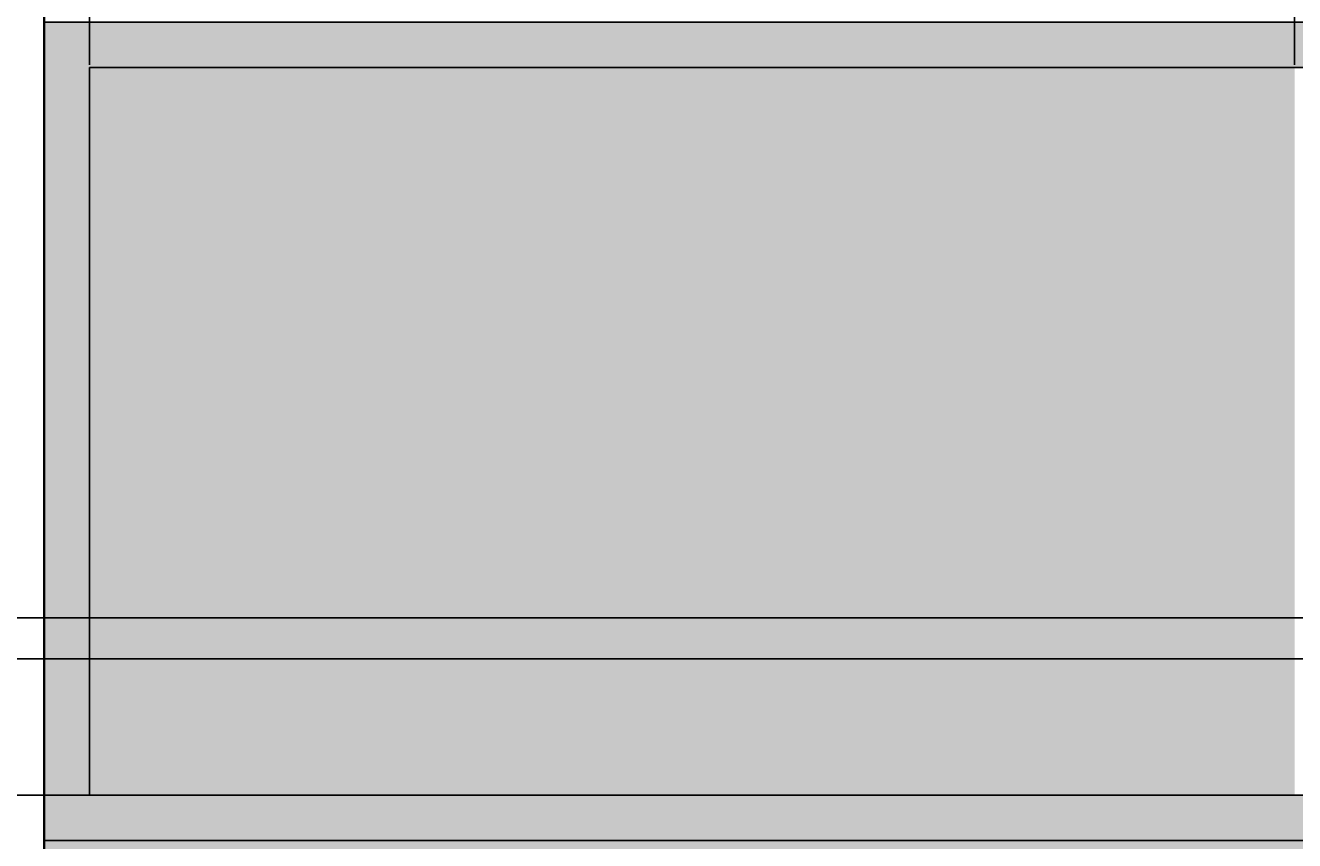
# Model space of a CAD drawing. Units: inches. Extents: x 4508 to 4723, y 847 to 1020.
# Tile 3 of 32: x 4550 to 4577, y 887 to 905. Entities that reach past the tile are written whole.
import ezdxf

# ---------------------------------------------------------------- set-up
doc = ezdxf.new("R2010")
doc.units = ezdxf.units.IN
for name, color, linetype, lineweight in [('A-ANNO-DIMS', 2, 'Continuous', 18), ('A-FURN', 8, 'Continuous', 25), ('A-WALL', 7, 'Continuous', 35), ('A-WALL-PATT', 254, 'Continuous', 13)]:
    doc.layers.add(name, color=color, linetype=linetype, lineweight=lineweight)
doc.styles.get("Standard").update_dxf_attribs({"font": 'arial.ttf'})
doc.dimstyles.get("Standard").update_dxf_attribs({"dimtxt": 0.18, "dimasz": 0.18, "dimexe": 0.18, "dimexo": 0.0625, "dimgap": 0.09, "dimtad": 0, "dimtih": 1, "dimtoh": 1, "dimdec": 4, "dimzin": 0, "dimdsep": 46, "dimtxsty": 'Standard', "dimcen": 0.09, "dimadec": 0, "dimazin": 0, "dimtfac": 1, "dimtdec": 4, "dimtofl": 0, "dimtmove": 0, "dimatfit": 3, "dimfxl": 1, "dimtolj": 1, "dimtzin": 0, "dimarcsym": 0})

# ---------------------------------------------------------------- blocks, each defined once
blk = doc.blocks.new('*D26')
at = {"layer": 'A-ANNO-DIMS', "color": 0, "lineweight": -2, "transparency": 16777216}
for p, q in [((4549.994, 904.809), (4549.994, 1002.877)), ((4550.994, 903.809), (4550.994, 1002.877)), ((4550.174, 1002.697), (4550.371, 1002.697)), ((4550.814, 1002.697), (4550.617, 1002.697))]:
    blk.add_line(p, q, dxfattribs=at)
at = {"layer": 'A-ANNO-DIMS', "color": 0, "lineweight": 9, "transparency": 16777216}
for points in [[(4550.174, 1002.727), (4550.174, 1002.667), (4549.994, 1002.697)], [(4550.814, 1002.727), (4550.814, 1002.667), (4550.994, 1002.697)]]:
    blk.add_solid(points, dxfattribs=at)
at = {"layer": 'Defpoints', "color": 0, "lineweight": 9, "transparency": 16777216}
for p in [(4550.994, 1002.697), (4549.994, 904.747), (4550.994, 903.747)]:
    blk.add_point(p, dxfattribs=at)
at = {"layer": 'A-ANNO-DIMS', "color": 0, "transparency": 16777216, "insert": (4550.494, 1002.697), "char_height": 0.18, "attachment_point": 5}
blk.add_mtext('\\A1;1', dxfattribs=at)
blk = doc.blocks.new('*D27')
at = {"layer": 'A-ANNO-DIMS', "color": 0, "lineweight": -2, "transparency": 16777216}
for p, q in [((4550.994, 903.809), (4550.994, 1002.877)), ((4577.494, 903.809), (4577.494, 1002.877)), ((4551.174, 1002.697), (4563.918, 1002.697)), ((4577.314, 1002.697), (4564.57, 1002.697))]:
    blk.add_line(p, q, dxfattribs=at)
at = {"layer": 'A-ANNO-DIMS', "color": 0, "lineweight": 9, "transparency": 16777216}
for points in [[(4551.174, 1002.727), (4551.174, 1002.667), (4550.994, 1002.697)], [(4577.314, 1002.727), (4577.314, 1002.667), (4577.494, 1002.697)]]:
    blk.add_solid(points, dxfattribs=at)
at = {"layer": 'Defpoints', "color": 0, "lineweight": 9, "transparency": 16777216}
for p in [(4577.494, 1002.697), (4550.994, 903.747), (4577.494, 903.747)]:
    blk.add_point(p, dxfattribs=at)
at = {"layer": 'A-ANNO-DIMS', "color": 0, "transparency": 16777216, "insert": (4564.244, 1002.697), "char_height": 0.18, "attachment_point": 5}
blk.add_mtext('\\A1;26.5', dxfattribs=at)
blk = doc.blocks.new('*D28')
at = {"layer": 'A-ANNO-DIMS', "color": 0, "lineweight": -2, "transparency": 16777216}
for p, q in [((4577.494, 903.809), (4577.494, 1002.877)), ((4577.994, 903.809), (4577.994, 1002.877)), ((4577.314, 1002.697), (4577.134, 1002.697)), ((4578.174, 1002.697), (4578.354, 1002.697))]:
    blk.add_line(p, q, dxfattribs=at)
at = {"layer": 'A-ANNO-DIMS', "color": 0, "lineweight": 9, "transparency": 16777216}
for points in [[(4577.314, 1002.727), (4577.314, 1002.667), (4577.494, 1002.697)], [(4578.174, 1002.727), (4578.174, 1002.667), (4577.994, 1002.697)]]:
    blk.add_solid(points, dxfattribs=at)
at = {"layer": 'Defpoints', "color": 0, "lineweight": 9, "transparency": 16777216}
for p in [(4577.994, 1002.697), (4577.494, 903.747), (4577.994, 903.747)]:
    blk.add_point(p, dxfattribs=at)
at = {"layer": 'A-ANNO-DIMS', "color": 0, "transparency": 16777216, "insert": (4578.608, 1002.697), "char_height": 0.18, "attachment_point": 5}
blk.add_mtext('\\A1;0.5', dxfattribs=at)
blk = doc.blocks.new('*D32')
at = {"layer": 'A-ANNO-DIMS', "color": 0, "lineweight": -2, "transparency": 16777216}
for p, q in [((4604.431, 890.747), (4532.864, 890.747)), ((4533.044, 890.567), (4533.044, 889.429)), ((4533.044, 887.927), (4533.044, 889.065)), ((4604.431, 887.747), (4532.864, 887.747))]:
    blk.add_line(p, q, dxfattribs=at)
at = {"layer": 'A-ANNO-DIMS', "color": 0, "lineweight": 9, "transparency": 16777216}
for points in [[(4533.014, 890.567), (4533.074, 890.567), (4533.044, 890.747)], [(4533.014, 887.927), (4533.074, 887.927), (4533.044, 887.747)]]:
    blk.add_solid(points, dxfattribs=at)
at = {"layer": 'Defpoints', "color": 0, "lineweight": 9, "transparency": 16777216}
for p in [(4533.044, 890.747), (4604.494, 890.747), (4604.494, 887.747)]:
    blk.add_point(p, dxfattribs=at)
at = {"layer": 'A-ANNO-DIMS', "color": 0, "transparency": 16777216, "insert": (4533.044, 889.247), "char_height": 0.18, "attachment_point": 5}
blk.add_mtext('\\A1;3', dxfattribs=at)
blk = doc.blocks.new('*D41')
at = {"layer": 'A-ANNO-DIMS', "color": 0, "lineweight": -2, "transparency": 16777216}
for p, q in [((4533.044, 891.643), (4533.044, 891.823)), ((4533.044, 891.823), (4533.224, 891.823)), ((4616.47, 891.643), (4532.864, 891.643)), ((4533.044, 890.927), (4533.044, 891.463)), ((4608.499, 890.747), (4532.864, 890.747))]:
    blk.add_line(p, q, dxfattribs=at)
at = {"layer": 'A-ANNO-DIMS', "color": 0, "lineweight": 9, "transparency": 16777216}
for points in [[(4533.014, 891.463), (4533.074, 891.463), (4533.044, 891.643)], [(4533.014, 890.927), (4533.074, 890.927), (4533.044, 890.747)]]:
    blk.add_solid(points, dxfattribs=at)
at = {"layer": 'Defpoints', "color": 0, "lineweight": 9, "transparency": 16777216}
for p in [(4533.044, 891.643), (4616.533, 891.643), (4608.562, 890.747)]:
    blk.add_point(p, dxfattribs=at)
at = {"layer": 'A-ANNO-DIMS', "color": 0, "transparency": 16777216, "insert": (4533.547, 891.823), "char_height": 0.18, "attachment_point": 5}
blk.add_mtext('\\A1;0.90', dxfattribs=at)

msp = doc.modelspace()

# ---------------------------------------------------------------- hatches: boundary and pattern name
at = {"layer": 'A-WALL-PATT', "transparency": 33554508}
h = msp.add_hatch(color=256, dxfattribs=at)
h.dxf.hatch_style = 1
h.paths.add_polyline_path([(4661.6706, 954.043, -0.3739004), (4658.5765, 957.6021, -1), (4665.7646, 957.6021, -0.3739004), (4662.6706, 954.043), (4662.6706, 944.4021, -0.2114781), (4670.3062, 945.0869), (4670.3062, 968.0592, -0.4632086), (4663.3246, 973.9783, -0.4632086), (4670.3062, 979.8975), (4670.3062, 994.7469), (4588.9938, 994.7469), (4588.9938, 904.7469), (4657.9938, 904.7469), (4657.9938, 886.7469), (4549.9938, 886.7469), (4549.9938, 878.7469), (4693.9938, 878.7469), (4693.9938, 994.7469), (4671.8062, 994.7469), (4671.8062, 979.4411, -0.2941682), (4675.3246, 973.9783, -0.2941682), (4671.8062, 968.5156), (4671.8062, 944.4278, -0.2741114), (4676.7298, 936.1217, -0.2741114), (4671.8062, 927.8155), (4671.8062, 907.6998, -0.3779645), (4677.0562, 901.7469, -0.3779645), (4671.8062, 895.7939), (4671.8062, 883.7469), (4670.3062, 883.7469), (4670.3062, 895.7939, -0.3779645), (4665.0562, 901.7469, -0.3779645), (4670.3062, 907.6998), (4670.3062, 927.1564, -0.2114781), (4662.6706, 927.8412), (4662.6706, 918.2003, -0.3739004), (4665.7646, 914.6412, -1), (4658.5765, 914.6412, -0.3739004), (4661.6706, 918.2003), (4661.6706, 928.4807, -0.2391825), (4657.7936, 936.1217, -0.2391825), (4661.6706, 943.7626)])
at = {"layer": 'A-WALL-PATT', "transparency": 33554681}
h = msp.add_hatch(color=256, dxfattribs=at)
h.dxf.hatch_style = 1
h.paths.add_polyline_path([(4577.4938, 903.7469), (4550.9938, 903.7469), (4550.9938, 887.7469), (4577.4938, 887.7469)], flags=0)
h.paths.add_polyline_path([(4603.9938, 903.7469), (4577.9938, 903.7469), (4577.9938, 887.7469), (4603.9938, 887.7469)], flags=0)
h.paths.add_polyline_path([(4656.9938, 903.7469), (4630.9938, 903.7469), (4630.9938, 887.7469), (4656.9938, 887.7469)], flags=0)
h.paths.add_polyline_path([(4657.9938, 904.7469), (4549.9938, 904.7469), (4549.9938, 886.7469), (4657.9938, 886.7469)])
h.paths.add_polyline_path([(4656.9938, 903.7469), (4656.9938, 887.7469), (4550.9938, 887.7469), (4550.9938, 903.7469)], flags=16)
h = msp.add_hatch(color=256, dxfattribs=at)
h.dxf.hatch_style = 1
h.paths.add_polyline_path([(4577.4938, 903.7469), (4550.9938, 903.7469), (4550.9938, 887.7469), (4577.4938, 887.7469)])
h.paths.add_polyline_path([(4603.9938, 903.7469), (4577.9938, 903.7469), (4577.9938, 887.7469), (4603.9938, 887.7469)])
h.paths.add_polyline_path([(4656.9938, 903.7469), (4630.9938, 903.7469), (4630.9938, 887.7469), (4656.9938, 887.7469)])

# ---------------------------------------------------------------- linework, layer by layer
at = {"layer": 'A-FURN'}
for points in [[(4657.9938, 886.7469), (4549.9938, 886.7469), (4549.9938, 904.7469), (4657.9938, 904.7469)], [(4656.9938, 887.7469), (4550.9938, 887.7469), (4550.9938, 903.7469), (4656.9938, 903.7469)]]:
    msp.add_lwpolyline(points, close=True, dxfattribs=at)
at = {"layer": 'A-WALL'}
msp.add_line((4549.9938, 874.7469), (4549.9938, 994.7469), dxfattribs=at)

# ---------------------------------------------------------------- dimensions: what is measured, and where the dimension line sits
at = {"layer": 'A-ANNO-DIMS'}
for base, p1, p2, override, picture, middle in [((4550.9938, 1002.6969), (4549.9938, 904.7469), (4550.9938, 903.7469), {"dimdec": 0, "dimlfac": 1, "dimrnd": 0, "dimzin": 0, "dimdsep": 46, "dimlunit": 2}, '*D26', (4550.4938, 1002.6969)), ((4577.4938, 1002.6969), (4550.9938, 903.7469), (4577.4938, 903.7469), {"dimdec": 1, "dimlfac": 1, "dimrnd": 0, "dimzin": 0, "dimdsep": 46, "dimlunit": 2}, '*D27', (4564.2438, 1002.6969)), ((4577.9938, 1002.6969), (4577.4938, 903.7469), (4577.9938, 903.7469), {"dimdec": 1, "dimlfac": 1, "dimrnd": 0, "dimzin": 0, "dimdsep": 46, "dimlunit": 2}, '*D28', (4578.6083, 1002.6969))]:
    dim = msp.add_linear_dim(base=base, p1=p1, p2=p2, dimstyle='Standard', override=override, dxfattribs=at)
    dim.commit()
    dim.dimension.update_dxf_attribs({"geometry": picture, "text_midpoint": middle})
for base, p1, p2, override, picture, middle in [((4533.0438, 891.6433), (4608.5617, 890.7469), (4616.5328, 891.6433), {"dimdec": 2, "dimlfac": 1, "dimrnd": 0, "dimzin": 0, "dimdsep": 46, "dimlunit": 2}, '*D41', (4533.5473, 891.8233)), ((4533.0438, 890.7469), (4604.4938, 887.7469), (4604.4938, 890.7469), {"dimdec": 0, "dimlfac": 1, "dimrnd": 0, "dimzin": 0, "dimdsep": 46, "dimlunit": 2}, '*D32', (4533.0438, 889.2469))]:
    dim = msp.add_linear_dim(base=base, p1=p1, p2=p2, angle=90, dimstyle='Standard', override=override, dxfattribs=at)
    dim.commit()
    dim.dimension.update_dxf_attribs({"geometry": picture, "text_midpoint": middle})

doc.saveas('drawing.dxf')
